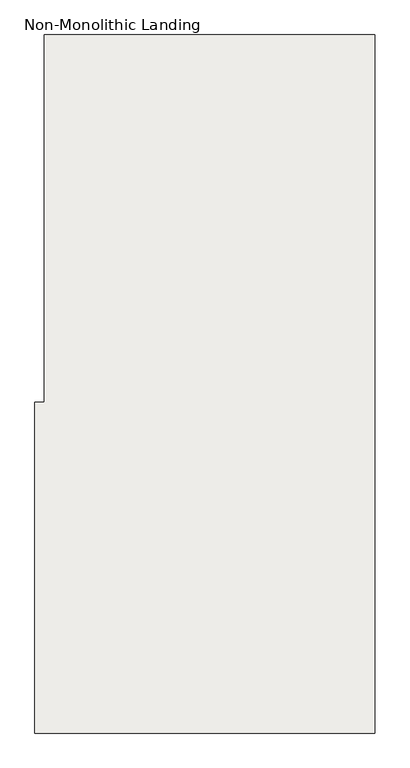
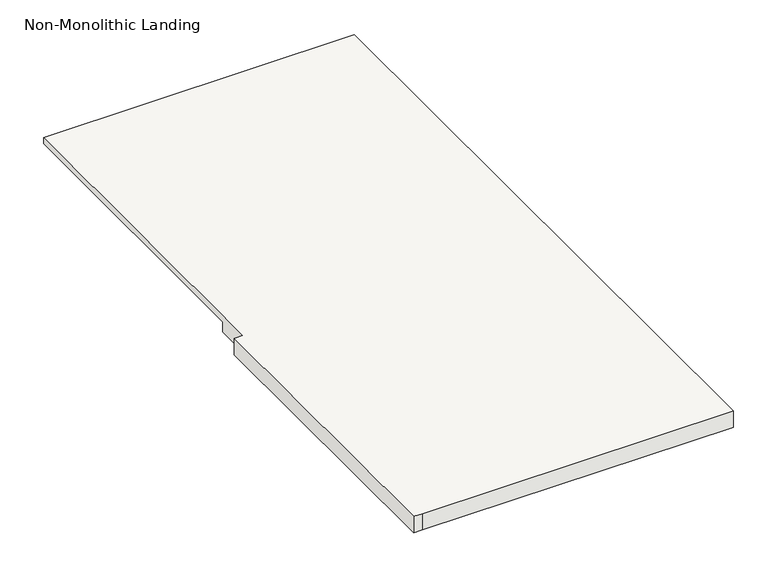
"""IFC4 building model written with IfcOpenShell, lengths in millimetres: slab geometry, Non-Monolithic Landing."""

from ifc_helpers import new_model, si_unit, origin, place, context, project, spatial, faceted_brep, source, transform, mapped, element, save


def non_monolithic_landing_4fb2f634(model_context):
    return source(origin(), model_context, "Body", "Brep", [
        faceted_brep([(923.4845537, -3822.9544725, 4781.55), (948.8845537, -3822.9544725, 4756.15), (948.8845537, -4737.3544725, 4756.15), (923.4845537, -4737.3544725, 4781.55), (923.4845537, -4838.9544725, 4800.6), (898.0845537, -4838.9544725, 4800.6), (898.0845537, -5753.3544725, 4800.6), (923.4845537, -5753.3544725, 4800.6), (1837.8845537, -5753.3544725, 4800.6), (1837.8845537, -3822.9544725, 4800.6), (923.4845537, -3822.9544725, 4800.6), (948.8845537, -4737.3544725, 4749.8), (948.8845537, -3822.9544725, 4749.8), (1837.8845537, -3822.9544725, 4749.8), (1837.8845537, -5753.3544725, 4749.8), (923.4845537, -5753.3544725, 4749.8), (898.0845537, -5753.3544725, 4749.8), (898.0845537, -4838.9544725, 4749.8), (923.4845537, -4838.9544725, 4749.8), (923.4845537, -4737.3544725, 4749.8)], [[[0, 1, 2, 3]], [[4, 5, 6, 7, 8, 9, 10]], [[11, 12, 13, 14, 15, 16, 17, 18, 19]], [[12, 11, 2, 1]], [[11, 19, 3, 2]], [[4, 10, 0, 3, 19, 18]], [[5, 4, 18, 17]], [[6, 5, 17, 16]], [[7, 6, 16, 15]], [[8, 7, 15, 14]], [[9, 8, 14, 13]], [[10, 9, 13, 12, 1, 0]]]),
    ])


if __name__ == "__main__":
    model = new_model("IFC4")
    model_context = context("Model", 3, world=origin())
    ifc_project = project(units=[si_unit("LENGTHUNIT", "METRE", prefix="MILLI")], contexts=[model_context])
    site = spatial("IfcSite", under=ifc_project)
    building = spatial("IfcBuilding", under=site)
    placement = place(None, origin())
    non_monolithic_landing_shape = non_monolithic_landing_4fb2f634(model_context)
    element("IfcSlab", 1, ObjectType="Non-Monolithic Landing", at=placement, inside=building, context=model_context, shape_type="MappedRepresentation", body=[
        mapped(non_monolithic_landing_shape, transform((0.0, 0.0, 0.0), x_axis=(1.0, 0.0, 0.0), y_axis=(0.0, 1.0, 0.0), z_axis=(0.0, 0.0, 1.0))),
    ])
    save(model, "model.ifc")
